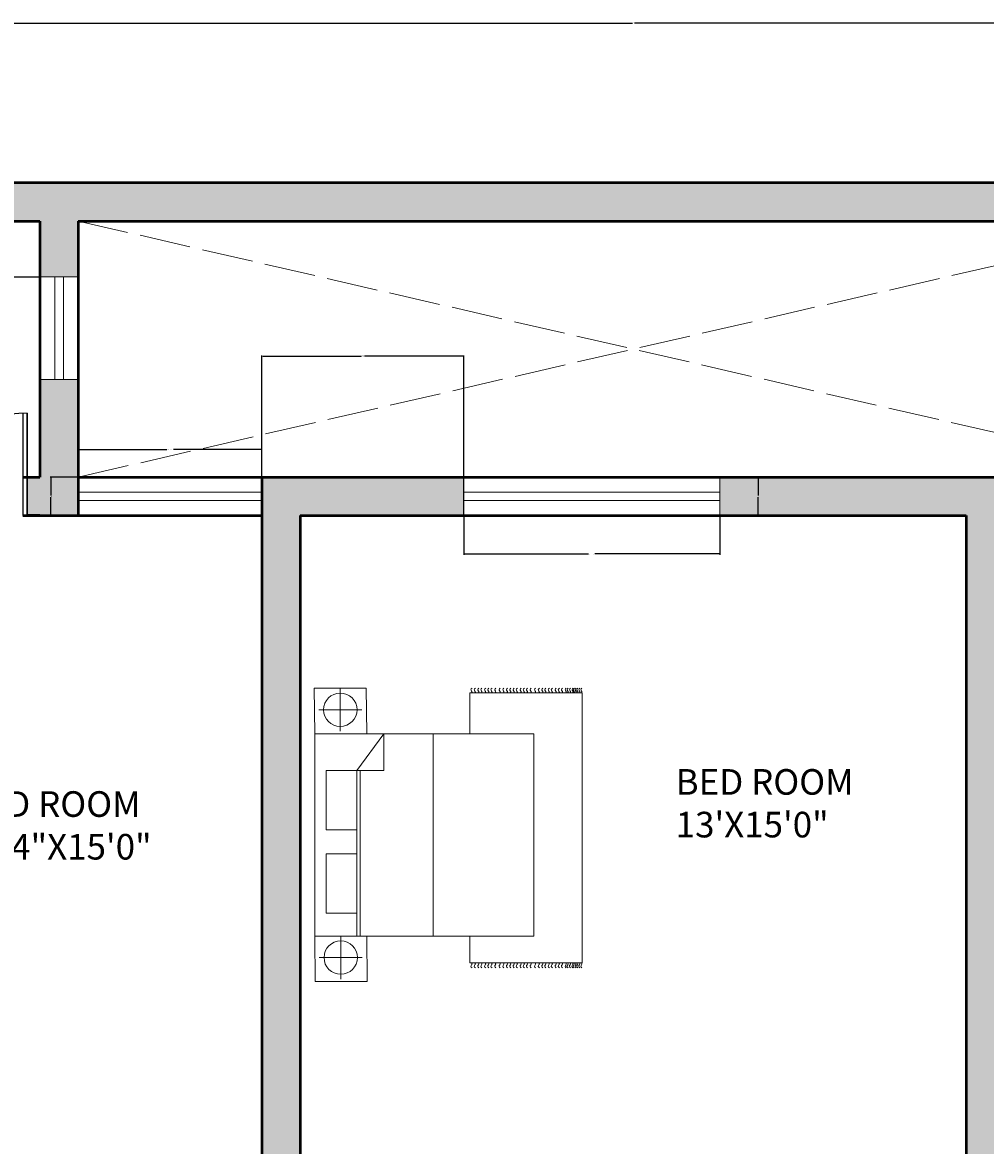
# Model space of a CAD drawing. Units: inches. Extents: x 383 to 970, y 275 to 1088.
# Tile 8 of 11: x 533 to 759, y 825 to 1088. Entities that reach past the tile are written whole.
import ezdxf

# ---------------------------------------------------------------- set-up
doc = ezdxf.new("R2010")
doc.units = ezdxf.units.IN
doc.header["$MEASUREMENT"] = 0
doc.linetypes.add('ACAD_ISO02W100', pattern=[15, 12, -3])
for name, color, linetype, lineweight in [('A-ANNO-DIMS', 2, 'Continuous', 18), ('A-AREA-IDEN', 7, 'Continuous', 18), ('A-DOOR', 3, 'Continuous', 25), ('A-FLOR-OPEN', 8, 'ACAD_ISO02W100', 13), ('A-FURN', 8, 'Continuous', 18), ('A-GLAZ', 4, 'Continuous', 18), ('A-WALL', 7, 'Continuous', 50)]:
    doc.layers.add(name, color=color, linetype=linetype, lineweight=lineweight)
doc.layers.add('A-WALL-PATT', color=251, linetype='Continuous', lineweight=13, true_color=0x636466)
doc.styles.get("Standard").update_dxf_attribs({"font": 'arial.ttf'})
doc.dimstyles.get("Standard").update_dxf_attribs({"dimtxt": 0.18, "dimasz": 0.18, "dimexe": 0.18, "dimexo": 0.0625, "dimgap": 0.09, "dimtad": 0, "dimtih": 1, "dimtoh": 1, "dimdec": 4, "dimzin": 0, "dimdsep": 46, "dimtxsty": 'Standard', "dimcen": 0.09, "dimadec": 0, "dimazin": 0, "dimtfac": 1, "dimtdec": 4, "dimtofl": 0, "dimtmove": 0, "dimatfit": 3, "dimfxl": 1, "dimtolj": 1, "dimtzin": 0, "dimarcsym": 0})

# ---------------------------------------------------------------- blocks, each defined once
blk = doc.blocks.new('BED-DOUBLE-WITH-NIGHTSTANDS')
for p, q in [((6.09, 68.68), (6.09, 58.62)), ((36.42, 67.59), (62.78, 67.59)), ((36.42, 58.05), (36.42, 67.59)), ((62.78, 67.59), (62.78, 4.35)), ((1.07, 63.65), (11.12, 63.65)), ((9.97, 49.39), (16.32, 58)), ((16.32, 49.44), (16.32, 58)), ((27.82, 58.05), (27.82, 10.63)), ((9.97, 49.44), (16.32, 49.44)), ((9.97, 49.39), (9.97, 10.63)), ((10.78, 49.44), (10.78, 10.63)), ((6.2, 10.63), (6.2, 0.57)), ((36.42, 4.35), (36.42, 10.65)), ((1.17, 5.6), (11.22, 5.6)), ((62.78, 4.35), (36.42, 4.35))]:
    blk.add_line(p, q)
for points in [[(12.29, 58.05), (12.19, 68.68), (0, 68.68), (0.1, 58.05)], [(0.1, 58.05), (51.42, 58.05), (51.42, 10.63), (0.1, 10.63)], [(2.8, 49.44), (9.97, 49.44), (9.97, 35.55), (2.8, 35.55)], [(2.8, 29.88), (9.97, 29.88), (9.97, 15.98), (2.8, 15.98)], [(12.39, 0), (12.29, 10.63), (0.1, 10.63), (0.21, 0)]]:
    blk.add_lwpolyline(points, close=True)
for centre in [(6.09, 63.65), (6.2, 5.6)]:
    blk.add_circle(centre, 3.92)
for points, knots in [([(36.95, 68.71), (36.83, 68.61), (36.59, 68.42), (36.83, 68.08), (37, 67.8), (36.89, 67.65), (36.85, 67.58)], [0, 0, 0, 0, 0.400747, 0.791423, 1.067667, 1.29709, 1.29709, 1.29709, 1.29709]), ([(37.73, 68.71), (37.61, 68.61), (37.37, 68.42), (37.61, 68.08), (37.78, 67.8), (37.67, 67.65), (37.62, 67.58)], [0, 0, 0, 0, 0.400747, 0.791423, 1.067667, 1.29709, 1.29709, 1.29709, 1.29709]), ([(38.54, 68.71), (38.42, 68.61), (38.18, 68.42), (38.42, 68.08), (38.59, 67.8), (38.49, 67.65), (38.44, 67.58)], [0, 0, 0, 0, 0.400747, 0.791423, 1.067667, 1.29709, 1.29709, 1.29709, 1.29709]), ([(39.27, 68.71), (39.15, 68.61), (38.91, 68.42), (39.15, 68.08), (39.32, 67.8), (39.22, 67.65), (39.17, 67.58)], [0, 0, 0, 0, 0.400747, 0.791423, 1.067667, 1.29709, 1.29709, 1.29709, 1.29709]), ([(40.15, 68.71), (40.03, 68.61), (39.79, 68.42), (40.03, 68.08), (40.21, 67.8), (40.1, 67.65), (40.05, 67.58)], [0, 0, 0, 0, 0.400747, 0.791423, 1.067667, 1.29709, 1.29709, 1.29709, 1.29709]), ([(40.91, 68.71), (40.78, 68.61), (40.54, 68.42), (40.78, 68.08), (40.96, 67.8), (40.85, 67.65), (40.8, 67.58)], [0, 0, 0, 0, 0.400747, 0.791423, 1.067667, 1.29709, 1.29709, 1.29709, 1.29709]), ([(41.63, 68.71), (41.51, 68.61), (41.27, 68.42), (41.51, 68.08), (41.69, 67.8), (41.58, 67.65), (41.53, 67.58)], [0, 0, 0, 0, 0.400747, 0.791423, 1.067667, 1.29709, 1.29709, 1.29709, 1.29709]), ([(42.52, 68.71), (42.39, 68.61), (42.16, 68.42), (42.39, 68.08), (42.57, 67.8), (42.46, 67.65), (42.41, 67.58)], [0, 0, 0, 0, 0.400747, 0.791423, 1.067667, 1.29709, 1.29709, 1.29709, 1.29709]), ([(43.55, 68.71), (43.43, 68.61), (43.19, 68.42), (43.43, 68.08), (43.6, 67.8), (43.5, 67.65), (43.45, 67.58)], [0, 0, 0, 0, 0.400747, 0.791423, 1.067667, 1.29709, 1.29709, 1.29709, 1.29709]), ([(44.43, 68.71), (44.31, 68.61), (44.07, 68.42), (44.31, 68.08), (44.49, 67.8), (44.38, 67.65), (44.33, 67.58)], [0, 0, 0, 0, 0.400747, 0.791423, 1.067667, 1.29709, 1.29709, 1.29709, 1.29709]), ([(45.25, 68.71), (45.13, 68.61), (44.89, 68.42), (45.13, 68.08), (45.3, 67.8), (45.2, 67.65), (45.15, 67.58)], [0, 0, 0, 0, 0.400747, 0.791423, 1.067667, 1.29709, 1.29709, 1.29709, 1.29709]), ([(46.03, 68.71), (45.91, 68.61), (45.67, 68.42), (45.91, 68.08), (46.08, 67.8), (45.97, 67.65), (45.92, 67.58)], [0, 0, 0, 0, 0.400747, 0.791423, 1.067667, 1.29709, 1.29709, 1.29709, 1.29709]), ([(46.84, 68.71), (46.72, 68.61), (46.48, 68.42), (46.72, 68.08), (46.9, 67.8), (46.79, 67.65), (46.74, 67.58)], [0, 0, 0, 0, 0.400747, 0.791423, 1.067667, 1.29709, 1.29709, 1.29709, 1.29709]), ([(47.57, 68.71), (47.45, 68.61), (47.21, 68.42), (47.45, 68.08), (47.62, 67.8), (47.52, 67.65), (47.47, 67.58)], [0, 0, 0, 0, 0.400747, 0.791423, 1.067667, 1.29709, 1.29709, 1.29709, 1.29709]), ([(48.45, 68.71), (48.33, 68.61), (48.09, 68.42), (48.33, 68.08), (48.51, 67.8), (48.4, 67.65), (48.35, 67.58)], [0, 0, 0, 0, 0.400747, 0.791423, 1.067667, 1.29709, 1.29709, 1.29709, 1.29709]), ([(49.21, 68.71), (49.08, 68.61), (48.85, 68.42), (49.08, 68.08), (49.26, 67.8), (49.15, 67.65), (49.1, 67.58)], [0, 0, 0, 0, 0.400747, 0.791423, 1.067667, 1.29709, 1.29709, 1.29709, 1.29709]), ([(49.93, 68.71), (49.81, 68.61), (49.57, 68.42), (49.81, 68.08), (49.99, 67.8), (49.88, 67.65), (49.83, 67.58)], [0, 0, 0, 0, 0.400747, 0.791423, 1.067667, 1.29709, 1.29709, 1.29709, 1.29709]), ([(50.82, 68.71), (50.69, 68.61), (50.46, 68.42), (50.69, 68.08), (50.87, 67.8), (50.76, 67.65), (50.71, 67.58)], [0, 0, 0, 0, 0.400747, 0.791423, 1.067667, 1.29709, 1.29709, 1.29709, 1.29709]), ([(51.85, 68.71), (51.73, 68.61), (51.49, 68.42), (51.73, 68.08), (51.9, 67.8), (51.8, 67.65), (51.75, 67.58)], [0, 0, 0, 0, 0.400747, 0.791423, 1.067667, 1.29709, 1.29709, 1.29709, 1.29709]), ([(52.74, 68.71), (52.61, 68.61), (52.37, 68.42), (52.61, 68.08), (52.79, 67.8), (52.68, 67.65), (52.63, 67.58)], [0, 0, 0, 0, 0.400747, 0.791423, 1.067667, 1.29709, 1.29709, 1.29709, 1.29709]), ([(53.55, 68.71), (53.43, 68.61), (53.19, 68.42), (53.43, 68.08), (53.6, 67.8), (53.5, 67.65), (53.45, 67.58)], [0, 0, 0, 0, 0.400747, 0.791423, 1.067667, 1.29709, 1.29709, 1.29709, 1.29709]), ([(54.24, 68.71), (54.12, 68.61), (53.88, 68.42), (54.12, 68.08), (54.29, 67.8), (54.19, 67.65), (54.14, 67.58)], [0, 0, 0, 0, 0.400747, 0.791423, 1.067667, 1.29709, 1.29709, 1.29709, 1.29709]), ([(55.06, 68.71), (54.94, 68.61), (54.7, 68.42), (54.94, 68.08), (55.11, 67.8), (55, 67.65), (54.95, 67.58)], [0, 0, 0, 0, 0.400747, 0.791423, 1.067667, 1.29709, 1.29709, 1.29709, 1.29709]), ([(55.78, 68.71), (55.66, 68.61), (55.42, 68.42), (55.66, 68.08), (55.84, 67.8), (55.73, 67.65), (55.68, 67.58)], [0, 0, 0, 0, 0.400747, 0.791423, 1.067667, 1.29709, 1.29709, 1.29709, 1.29709]), ([(56.67, 68.71), (56.55, 68.61), (56.31, 68.42), (56.55, 68.08), (56.72, 67.8), (56.61, 67.65), (56.56, 67.58)], [0, 0, 0, 0, 0.400747, 0.791423, 1.067667, 1.29709, 1.29709, 1.29709, 1.29709]), ([(57.42, 68.71), (57.3, 68.61), (57.06, 68.42), (57.3, 68.08), (57.47, 67.8), (57.36, 67.65), (57.32, 67.58)], [0, 0, 0, 0, 0.400747, 0.791423, 1.067667, 1.29709, 1.29709, 1.29709, 1.29709]), ([(58.15, 68.71), (58.03, 68.61), (57.79, 68.42), (58.03, 68.08), (58.2, 67.8), (58.1, 67.66), (58.05, 67.59)], [0, 0, 0, 0, 0.400747, 0.791423, 1.067667, 1.283686, 1.283686, 1.283686, 1.283686]), ([(59.03, 68.71), (58.91, 68.61), (58.67, 68.42), (58.91, 68.08), (59.08, 67.8), (58.98, 67.66), (58.93, 67.59)], [0, 0, 0, 0, 0.400747, 0.791423, 1.067667, 1.283686, 1.283686, 1.283686, 1.283686]), ([(59.46, 68.71), (59.34, 68.61), (59.09, 68.42), (59.34, 68.08), (59.51, 67.8), (59.41, 67.66), (59.36, 67.59)], [0, 0, 0, 0, 0.402903, 0.794912, 1.071156, 1.287177, 1.287177, 1.287177, 1.287177]), ([(60.05, 68.71), (59.93, 68.61), (59.69, 68.42), (59.93, 68.08), (60.1, 67.8), (60, 67.66), (59.96, 67.59)], [0, 0, 0, 0, 0.400747, 0.791423, 1.067667, 1.283686, 1.283686, 1.283686, 1.283686]), ([(60.63, 68.71), (60.51, 68.61), (60.27, 68.42), (60.51, 68.08), (60.68, 67.8), (60.58, 67.66), (60.53, 67.59)], [0, 0, 0, 0, 0.400747, 0.791423, 1.067667, 1.283686, 1.283686, 1.283686, 1.283686]), ([(60.94, 68.71), (60.82, 68.61), (60.58, 68.42), (60.81, 68.08), (60.99, 67.8), (60.89, 67.66), (60.84, 67.59)], [0, 0, 0, 0, 0.400747, 0.791423, 1.067667, 1.283686, 1.283686, 1.283686, 1.283686]), ([(61.36, 68.71), (61.23, 68.61), (60.99, 68.42), (61.23, 68.08), (61.41, 67.8), (61.3, 67.65), (61.25, 67.58)], [0, 0, 0, 0, 0.400747, 0.791423, 1.067667, 1.29709, 1.29709, 1.29709, 1.29709]), ([(61.75, 68.71), (61.63, 68.61), (61.39, 68.42), (61.63, 68.08), (61.8, 67.8), (61.7, 67.65), (61.65, 67.58)], [0, 0, 0, 0, 0.400747, 0.791423, 1.067667, 1.29709, 1.29709, 1.29709, 1.29709]), ([(62.24, 68.71), (62.12, 68.61), (61.88, 68.42), (62.12, 68.08), (62.29, 67.8), (62.18, 67.65), (62.13, 67.58)], [0, 0, 0, 0, 0.400747, 0.791423, 1.067667, 1.29709, 1.29709, 1.29709, 1.29709]), ([(62.71, 68.71), (62.59, 68.61), (62.35, 68.42), (62.59, 68.08), (62.76, 67.8), (62.66, 67.65), (62.61, 67.58)], [0, 0, 0, 0, 0.400747, 0.791423, 1.067667, 1.29709, 1.29709, 1.29709, 1.29709]), ([(36.95, 3.23), (36.83, 3.32), (36.59, 3.52), (36.83, 3.86), (37, 4.14), (36.89, 4.29), (36.85, 4.35)], [0, 0, 0, 0, 0.400747, 0.791423, 1.067667, 1.29709, 1.29709, 1.29709, 1.29709]), ([(37.73, 3.23), (37.61, 3.32), (37.37, 3.52), (37.61, 3.86), (37.78, 4.14), (37.67, 4.29), (37.62, 4.35)], [0, 0, 0, 0, 0.400747, 0.791423, 1.067667, 1.29709, 1.29709, 1.29709, 1.29709]), ([(38.54, 3.23), (38.42, 3.32), (38.18, 3.52), (38.42, 3.86), (38.59, 4.14), (38.49, 4.29), (38.44, 4.35)], [0, 0, 0, 0, 0.400747, 0.791423, 1.067667, 1.29709, 1.29709, 1.29709, 1.29709]), ([(39.27, 3.23), (39.15, 3.32), (38.91, 3.52), (39.15, 3.86), (39.32, 4.14), (39.22, 4.29), (39.17, 4.35)], [0, 0, 0, 0, 0.400747, 0.791423, 1.067667, 1.29709, 1.29709, 1.29709, 1.29709]), ([(40.15, 3.23), (40.03, 3.32), (39.79, 3.52), (40.03, 3.86), (40.21, 4.14), (40.1, 4.29), (40.05, 4.35)], [0, 0, 0, 0, 0.400747, 0.791423, 1.067667, 1.29709, 1.29709, 1.29709, 1.29709]), ([(40.91, 3.23), (40.78, 3.32), (40.54, 3.52), (40.78, 3.86), (40.96, 4.14), (40.85, 4.29), (40.8, 4.35)], [0, 0, 0, 0, 0.400747, 0.791423, 1.067667, 1.29709, 1.29709, 1.29709, 1.29709]), ([(41.63, 3.23), (41.51, 3.32), (41.27, 3.52), (41.51, 3.86), (41.69, 4.14), (41.58, 4.29), (41.53, 4.35)], [0, 0, 0, 0, 0.400747, 0.791423, 1.067667, 1.29709, 1.29709, 1.29709, 1.29709]), ([(42.52, 3.23), (42.39, 3.32), (42.16, 3.52), (42.39, 3.86), (42.57, 4.14), (42.46, 4.29), (42.41, 4.35)], [0, 0, 0, 0, 0.400747, 0.791423, 1.067667, 1.29709, 1.29709, 1.29709, 1.29709]), ([(43.55, 3.23), (43.43, 3.32), (43.19, 3.52), (43.43, 3.86), (43.6, 4.14), (43.5, 4.29), (43.45, 4.35)], [0, 0, 0, 0, 0.400747, 0.791423, 1.067667, 1.29709, 1.29709, 1.29709, 1.29709]), ([(44.43, 3.23), (44.31, 3.32), (44.07, 3.52), (44.31, 3.86), (44.49, 4.14), (44.38, 4.29), (44.33, 4.35)], [0, 0, 0, 0, 0.400747, 0.791423, 1.067667, 1.29709, 1.29709, 1.29709, 1.29709]), ([(45.25, 3.23), (45.13, 3.32), (44.89, 3.52), (45.13, 3.86), (45.3, 4.14), (45.2, 4.29), (45.15, 4.35)], [0, 0, 0, 0, 0.400747, 0.791423, 1.067667, 1.29709, 1.29709, 1.29709, 1.29709]), ([(46.03, 3.23), (45.91, 3.32), (45.67, 3.52), (45.91, 3.86), (46.08, 4.14), (45.97, 4.29), (45.92, 4.35)], [0, 0, 0, 0, 0.400747, 0.791423, 1.067667, 1.29709, 1.29709, 1.29709, 1.29709]), ([(46.84, 3.23), (46.72, 3.32), (46.48, 3.52), (46.72, 3.86), (46.9, 4.14), (46.79, 4.29), (46.74, 4.35)], [0, 0, 0, 0, 0.400747, 0.791423, 1.067667, 1.29709, 1.29709, 1.29709, 1.29709]), ([(47.57, 3.23), (47.45, 3.32), (47.21, 3.52), (47.45, 3.86), (47.62, 4.14), (47.52, 4.29), (47.47, 4.35)], [0, 0, 0, 0, 0.400747, 0.791423, 1.067667, 1.29709, 1.29709, 1.29709, 1.29709]), ([(48.45, 3.23), (48.33, 3.32), (48.09, 3.52), (48.33, 3.86), (48.51, 4.14), (48.4, 4.29), (48.35, 4.35)], [0, 0, 0, 0, 0.400747, 0.791423, 1.067667, 1.29709, 1.29709, 1.29709, 1.29709]), ([(49.21, 3.23), (49.08, 3.32), (48.85, 3.52), (49.08, 3.86), (49.26, 4.14), (49.15, 4.29), (49.1, 4.35)], [0, 0, 0, 0, 0.400747, 0.791423, 1.067667, 1.29709, 1.29709, 1.29709, 1.29709]), ([(49.93, 3.23), (49.81, 3.32), (49.57, 3.52), (49.81, 3.86), (49.99, 4.14), (49.88, 4.29), (49.83, 4.35)], [0, 0, 0, 0, 0.400747, 0.791423, 1.067667, 1.29709, 1.29709, 1.29709, 1.29709]), ([(50.82, 3.23), (50.69, 3.32), (50.46, 3.52), (50.69, 3.86), (50.87, 4.14), (50.76, 4.29), (50.71, 4.35)], [0, 0, 0, 0, 0.400747, 0.791423, 1.067667, 1.29709, 1.29709, 1.29709, 1.29709]), ([(51.85, 3.23), (51.73, 3.32), (51.49, 3.52), (51.73, 3.86), (51.9, 4.14), (51.8, 4.29), (51.75, 4.35)], [0, 0, 0, 0, 0.400747, 0.791423, 1.067667, 1.29709, 1.29709, 1.29709, 1.29709]), ([(52.74, 3.23), (52.61, 3.32), (52.37, 3.52), (52.61, 3.86), (52.79, 4.14), (52.68, 4.29), (52.63, 4.35)], [0, 0, 0, 0, 0.400747, 0.791423, 1.067667, 1.29709, 1.29709, 1.29709, 1.29709]), ([(53.55, 3.23), (53.43, 3.32), (53.19, 3.52), (53.43, 3.86), (53.6, 4.14), (53.5, 4.29), (53.45, 4.35)], [0, 0, 0, 0, 0.400747, 0.791423, 1.067667, 1.29709, 1.29709, 1.29709, 1.29709]), ([(54.24, 3.23), (54.12, 3.32), (53.88, 3.52), (54.12, 3.86), (54.29, 4.14), (54.19, 4.29), (54.14, 4.35)], [0, 0, 0, 0, 0.400747, 0.791423, 1.067667, 1.29709, 1.29709, 1.29709, 1.29709]), ([(55.06, 3.23), (54.94, 3.32), (54.7, 3.52), (54.94, 3.86), (55.11, 4.14), (55, 4.29), (54.95, 4.35)], [0, 0, 0, 0, 0.400747, 0.791423, 1.067667, 1.29709, 1.29709, 1.29709, 1.29709]), ([(55.78, 3.23), (55.66, 3.32), (55.42, 3.52), (55.66, 3.86), (55.84, 4.14), (55.73, 4.29), (55.68, 4.35)], [0, 0, 0, 0, 0.400747, 0.791423, 1.067667, 1.29709, 1.29709, 1.29709, 1.29709]), ([(56.67, 3.23), (56.55, 3.32), (56.31, 3.52), (56.55, 3.86), (56.72, 4.14), (56.61, 4.29), (56.56, 4.35)], [0, 0, 0, 0, 0.400747, 0.791423, 1.067667, 1.29709, 1.29709, 1.29709, 1.29709]), ([(57.42, 3.23), (57.3, 3.32), (57.06, 3.52), (57.3, 3.86), (57.47, 4.14), (57.36, 4.29), (57.32, 4.35)], [0, 0, 0, 0, 0.400747, 0.791423, 1.067667, 1.29709, 1.29709, 1.29709, 1.29709]), ([(58.15, 3.23), (58.03, 3.32), (57.79, 3.52), (58.03, 3.86), (58.2, 4.14), (58.09, 4.29), (58.04, 4.35)], [0, 0, 0, 0, 0.400747, 0.791423, 1.067667, 1.29709, 1.29709, 1.29709, 1.29709]), ([(59.03, 3.23), (58.91, 3.32), (58.67, 3.52), (58.91, 3.86), (59.08, 4.14), (58.98, 4.29), (58.93, 4.35)], [0, 0, 0, 0, 0.400747, 0.791423, 1.067667, 1.29709, 1.29709, 1.29709, 1.29709]), ([(59.46, 3.23), (59.33, 3.32), (59.08, 3.52), (59.34, 3.86), (59.51, 4.14), (59.4, 4.29), (59.36, 4.35)], [0, 0, 0, 0, 0.407265, 0.802015, 1.07826, 1.307683, 1.307683, 1.307683, 1.307683]), ([(60.03, 3.23), (59.9, 3.32), (59.67, 3.52), (59.9, 3.86), (60.08, 4.14), (59.97, 4.29), (59.92, 4.35)], [0, 0, 0, 0, 0.400747, 0.791423, 1.067667, 1.29709, 1.29709, 1.29709, 1.29709]), ([(60.6, 3.23), (60.48, 3.32), (60.24, 3.52), (60.48, 3.86), (60.65, 4.14), (60.54, 4.29), (60.5, 4.35)], [0, 0, 0, 0, 0.400747, 0.791423, 1.067667, 1.29709, 1.29709, 1.29709, 1.29709]), ([(60.91, 3.23), (60.79, 3.32), (60.55, 3.52), (60.79, 3.86), (60.96, 4.14), (60.85, 4.29), (60.81, 4.35)], [0, 0, 0, 0, 0.400747, 0.791423, 1.067667, 1.29709, 1.29709, 1.29709, 1.29709]), ([(61.33, 3.23), (61.21, 3.32), (60.97, 3.52), (61.21, 3.86), (61.38, 4.14), (61.27, 4.29), (61.22, 4.35)], [0, 0, 0, 0, 0.400747, 0.791423, 1.067667, 1.29709, 1.29709, 1.29709, 1.29709]), ([(61.72, 3.23), (61.6, 3.32), (61.36, 3.52), (61.6, 3.86), (61.78, 4.14), (61.67, 4.29), (61.62, 4.35)], [0, 0, 0, 0, 0.400747, 0.791423, 1.067667, 1.29709, 1.29709, 1.29709, 1.29709]), ([(62.21, 3.23), (62.09, 3.32), (61.85, 3.52), (62.09, 3.86), (62.26, 4.14), (62.16, 4.29), (62.11, 4.35)], [0, 0, 0, 0, 0.400747, 0.791423, 1.067667, 1.29709, 1.29709, 1.29709, 1.29709]), ([(62.71, 3.23), (62.59, 3.32), (62.35, 3.52), (62.59, 3.86), (62.76, 4.14), (62.66, 4.29), (62.61, 4.35)], [0, 0, 0, 0, 0.400747, 0.791423, 1.067667, 1.29709, 1.29709, 1.29709, 1.29709])]:
    blk.add_open_spline(points, degree=3, knots=knots)
blk = doc.blocks.new('DOOR-LEAF-24IN')
for p, q in [((23, 24), (23, 0)), ((24, 0), (24, 24)), ((24, 0), (23, 0))]:
    blk.add_line(p, q)
blk.add_arc((24, -2.7), 26.7, 90, 154.0108)
blk = doc.blocks.new('WIN-VENT-24IN')
for p, q in [((0, 0), (0, 24)), ((3.5, 0), (3.5, 24)), ((5.5, 24), (5.5, 0)), ((9, 24), (9, 0))]:
    blk.add_line(p, q)
blk = doc.blocks.new('WIN-60IN')
for p, q in [((60, 9), (0, 9)), ((60, 5.5), (0, 5.5)), ((0, 3.5), (60, 3.5)), ((0, 0), (60, 0))]:
    blk.add_line(p, q)
blk = doc.blocks.new('WIN-43IN')
for p, q in [((43, 9), (0, 9)), ((43, 5.5), (0, 5.5)), ((0, 3.5), (43, 3.5)), ((0, 0), (43, 0))]:
    blk.add_line(p, q)
blk = doc.blocks.new('*D21')
at = {"layer": 'A-ANNO-DIMS', "color": 0, "lineweight": -2, "transparency": 16777216}
for p, q in [((636.51, 972.07), (636.51, 962.96)), ((696.51, 972.07), (696.51, 962.96)), ((636.69, 963.14), (665.75, 963.14)), ((696.33, 963.14), (667.26, 963.14))]:
    blk.add_line(p, q, dxfattribs=at)
at = {"layer": 'A-ANNO-DIMS', "color": 0, "transparency": 16777216}
for points in [[(636.69, 963.17), (636.69, 963.11), (636.51, 963.14)], [(696.33, 963.17), (696.33, 963.11), (696.51, 963.14)]]:
    blk.add_solid(points, dxfattribs=at)
at = {"layer": 'Defpoints', "color": 0, "transparency": 16777216}
for p in [(636.51, 972.14), (696.51, 972.14), (696.51, 963.14)]:
    blk.add_point(p, dxfattribs=at)
at = {"layer": 'A-ANNO-DIMS', "color": 0, "transparency": 16777216, "insert": (666.51, 963.14), "char_height": 0.18, "attachment_point": 5}
blk.add_mtext('\\A1;W1 60 TYP.', dxfattribs=at)
blk = doc.blocks.new('*D22')
at = {"layer": 'A-ANNO-DIMS', "color": 0, "lineweight": -2, "transparency": 16777216}
for p, q in [((696.57, 981.14), (705.69, 981.14)), ((705.51, 980.96), (705.51, 976.82)), ((705.51, 972.32), (705.51, 976.45)), ((696.57, 972.14), (705.69, 972.14))]:
    blk.add_line(p, q, dxfattribs=at)
at = {"layer": 'A-ANNO-DIMS', "color": 0, "transparency": 16777216}
for points in [[(705.48, 980.96), (705.54, 980.96), (705.51, 981.14)], [(705.48, 972.32), (705.54, 972.32), (705.51, 972.14)]]:
    blk.add_solid(points, dxfattribs=at)
at = {"layer": 'Defpoints', "color": 0, "transparency": 16777216}
for p in [(696.51, 981.14), (705.51, 981.14), (696.51, 972.14)]:
    blk.add_point(p, dxfattribs=at)
at = {"layer": 'A-ANNO-DIMS', "color": 0, "transparency": 16777216, "insert": (705.51, 976.64), "char_height": 0.18, "attachment_point": 5}
blk.add_mtext('\\A1;9 TYP.', dxfattribs=at)
blk = doc.blocks.new('*D23')
at = {"layer": 'A-ANNO-DIMS', "color": 0, "lineweight": -2, "transparency": 16777216}
for p, q in [((546.24, 981.2), (546.24, 987.77)), ((546.42, 987.59), (566.98, 987.59)), ((589.06, 987.59), (568.5, 987.59)), ((589.24, 981.2), (589.24, 987.77))]:
    blk.add_line(p, q, dxfattribs=at)
at = {"layer": 'A-ANNO-DIMS', "color": 0, "transparency": 16777216}
for points in [[(546.42, 987.62), (546.42, 987.56), (546.24, 987.59)], [(589.06, 987.62), (589.06, 987.56), (589.24, 987.59)]]:
    blk.add_solid(points, dxfattribs=at)
at = {"layer": 'Defpoints', "color": 0, "transparency": 16777216}
for p in [(589.24, 987.59), (546.24, 981.14), (589.24, 981.14)]:
    blk.add_point(p, dxfattribs=at)
at = {"layer": 'A-ANNO-DIMS', "color": 0, "transparency": 16777216, "insert": (567.74, 987.59), "char_height": 0.18, "attachment_point": 5}
blk.add_mtext('\\A1;W2 43 TYP.', dxfattribs=at)
blk = doc.blocks.new('*D24')
at = {"layer": 'A-ANNO-DIMS', "color": 0, "lineweight": -2, "transparency": 16777216}
for p, q in [((546.18, 981.14), (539.61, 981.14)), ((539.79, 980.96), (539.79, 976.82)), ((539.79, 972.32), (539.79, 976.45)), ((546.18, 972.14), (539.61, 972.14))]:
    blk.add_line(p, q, dxfattribs=at)
at = {"layer": 'A-ANNO-DIMS', "color": 0, "transparency": 16777216}
for points in [[(539.76, 980.96), (539.82, 980.96), (539.79, 981.14)], [(539.76, 972.32), (539.82, 972.32), (539.79, 972.14)]]:
    blk.add_solid(points, dxfattribs=at)
at = {"layer": 'Defpoints', "color": 0, "transparency": 16777216}
for p in [(539.79, 981.14), (546.24, 981.14), (546.24, 972.14)]:
    blk.add_point(p, dxfattribs=at)
at = {"layer": 'A-ANNO-DIMS', "color": 0, "transparency": 16777216, "insert": (539.79, 976.64), "char_height": 0.18, "attachment_point": 5}
blk.add_mtext('\\A1;9 TYP.', dxfattribs=at)
blk = doc.blocks.new('*D37')
at = {"layer": 'A-ANNO-DIMS', "color": 0, "lineweight": -2, "transparency": 16777216}
for p, q in [((420.24, 1050.2), (420.24, 1087.67)), ((420.42, 1087.49), (675.95, 1087.49)), ((932.06, 1087.49), (676.53, 1087.49)), ((932.24, 1050.2), (932.24, 1087.67))]:
    blk.add_line(p, q, dxfattribs=at)
at = {"layer": 'A-ANNO-DIMS', "color": 0, "transparency": 16777216}
for points in [[(420.42, 1087.52), (420.42, 1087.46), (420.24, 1087.49)], [(932.06, 1087.52), (932.06, 1087.46), (932.24, 1087.49)]]:
    blk.add_solid(points, dxfattribs=at)
at = {"layer": 'Defpoints', "color": 0, "transparency": 16777216}
for p in [(932.24, 1087.49), (420.24, 1050.14), (932.24, 1050.14)]:
    blk.add_point(p, dxfattribs=at)
at = {"layer": 'A-ANNO-DIMS', "color": 0, "transparency": 16777216, "insert": (676.24, 1087.49), "char_height": 0.18, "attachment_point": 5}
blk.add_mtext('\\A1;512', dxfattribs=at)
blk = doc.blocks.new('*D52')
at = {"layer": 'A-ANNO-DIMS', "color": 0, "lineweight": -2, "transparency": 16777216}
for p, q in [((589.24, 972.2), (589.24, 1009.67)), ((589.42, 1009.49), (612.48, 1009.49)), ((636.33, 1009.49), (613.27, 1009.49)), ((636.51, 972.2), (636.51, 1009.67))]:
    blk.add_line(p, q, dxfattribs=at)
at = {"layer": 'A-ANNO-DIMS', "color": 0, "transparency": 16777216}
for points in [[(589.42, 1009.52), (589.42, 1009.46), (589.24, 1009.49)], [(636.33, 1009.52), (636.33, 1009.46), (636.51, 1009.49)]]:
    blk.add_solid(points, dxfattribs=at)
at = {"layer": 'Defpoints', "color": 0, "transparency": 16777216}
for p in [(636.51, 1009.49), (589.24, 972.14), (636.51, 972.14)]:
    blk.add_point(p, dxfattribs=at)
at = {"layer": 'A-ANNO-DIMS', "color": 0, "transparency": 16777216, "insert": (612.87, 1009.49), "char_height": 0.18, "attachment_point": 5}
blk.add_mtext('\\A1;47.27', dxfattribs=at)
blk = doc.blocks.new('*D62')
at = {"layer": 'A-ANNO-DIMS', "color": 0, "lineweight": -2, "transparency": 16777216}
for p, q in [((537.18, 1041.14), (499.71, 1041.14)), ((499.89, 1040.96), (499.89, 1034.77)), ((499.89, 1028.21), (499.89, 1034.4)), ((537.18, 1028.03), (499.71, 1028.03))]:
    blk.add_line(p, q, dxfattribs=at)
at = {"layer": 'A-ANNO-DIMS', "color": 0, "transparency": 16777216}
for points in [[(499.86, 1040.96), (499.92, 1040.96), (499.89, 1041.14)], [(499.86, 1028.21), (499.92, 1028.21), (499.89, 1028.03)]]:
    blk.add_solid(points, dxfattribs=at)
at = {"layer": 'Defpoints', "color": 0, "transparency": 16777216}
for p in [(499.89, 1041.14), (537.24, 1041.14), (537.24, 1028.03)]:
    blk.add_point(p, dxfattribs=at)
at = {"layer": 'A-ANNO-DIMS', "color": 0, "transparency": 16777216, "insert": (499.89, 1034.59), "char_height": 0.18, "attachment_point": 5}
blk.add_mtext('\\A1;13.103', dxfattribs=at)

msp = doc.modelspace()

# ---------------------------------------------------------------- hatches: boundary and pattern name
at = {"layer": 'A-WALL-PATT'}
h = msp.add_hatch(color=256, dxfattribs=at)
h.dxf.hatch_style = 1
h.paths.add_polyline_path([(651.24, 321.1365), (651.24, 417.1365), (735.24, 417.1365), (735.24, 491.9233), (726.24, 491.9233), (726.24, 426.1365), (582.24, 426.1365), (582.24, 606.1365), (687.24, 606.1365), (687.24, 615.1365), (573.24, 615.1365), (573.24, 546.1365), (570.24, 546.1365), (570.24, 537.1365), (573.24, 537.1365), (573.24, 414.1365), (582.24, 414.1365), (582.24, 417.1365), (642.24, 417.1365), (642.24, 321.1365), (621.6203, 321.1365), (621.6203, 312.1365), (651.24, 312.1365)], flags=17)
h.paths.add_polyline_path([(597.6203, 321.1365), (582.24, 321.1365), (582.24, 390.1365), (573.24, 390.1365), (573.24, 321.1365), (570.24, 321.1365), (570.24, 312.1365), (573.24, 312.1365), (597.6203, 312.1365)], flags=16)
h.paths.add_polyline_path([(534.24, 321.1365), (500.8868, 321.1365), (500.8868, 312.1365), (534.24, 312.1365)], flags=17)
h.paths.add_polyline_path([(735.24, 606.1365), (738.24, 606.1365), (738.24, 615.1365), (723.24, 615.1365), (723.24, 606.1365), (726.24, 606.1365), (726.24, 551.9233), (735.24, 551.9233)], flags=17)
h.paths.add_polyline_path([(848.0899, 615.1365), (814.24, 615.1365), (814.24, 689.38), (805.24, 689.38), (805.24, 615.1365), (802.24, 615.1365), (802.24, 606.1365), (848.0899, 606.1365)], flags=17)
h.paths.add_polyline_path([(530.24, 615.1365), (498.24, 615.1365), (498.24, 646.5351), (489.24, 646.5351), (489.24, 615.1365), (466.771, 615.1365), (466.771, 606.1365), (521.24, 606.1365), (521.24, 603.1365), (530.24, 603.1365), (530.24, 606.1365)], flags=17)
h.paths.add_polyline_path([(498.24, 744.1365), (489.24, 744.1365), (489.24, 706.5351), (498.24, 706.5351)], flags=17)
h.paths.add_polyline_path([(715.24, 792.1365), (598.24, 792.1365), (598.24, 972.1365), (636.5058, 972.1365), (636.5058, 981.1365), (589.24, 981.1365), (589.24, 972.1365), (589.24, 792.1365), (586.24, 792.1365), (586.24, 783.1365), (589.24, 783.1365), (715.24, 783.1365)], flags=17)
h.paths.add_polyline_path([(763.24, 981.1365), (696.5058, 981.1365), (696.5058, 972.1365), (754.24, 972.1365), (754.24, 792.1365), (751.24, 792.1365), (751.24, 783.1365), (754.24, 783.1365), (764.24, 783.1365), (764.24, 792.1365), (763.24, 792.1365)], flags=17)
h.paths.add_polyline_path([(815.24, 1001.9492), (806.24, 1001.9492), (806.24, 972.1365), (818.24, 972.1365), (818.24, 981.1365), (815.24, 981.1365)], flags=17)
h.paths.add_polyline_path([(546.24, 1004.0336), (537.24, 1004.0336), (537.24, 981.1365), (534.24, 981.1365), (534.24, 972.1365), (537.24, 972.1365), (546.24, 972.1365), (546.24, 981.1365)], flags=17)
h.paths.add_polyline_path([(884.0899, 606.1365), (932.24, 606.1365), (932.24, 1050.1365), (420.24, 1050.1365), (420.24, 312.1365), (440.8868, 312.1365), (440.8868, 321.1365), (429.24, 321.1365), (429.24, 537.1365), (538.24, 537.1365), (538.24, 546.1365), (530.24, 546.1365), (530.24, 579.1365), (521.24, 579.1365), (521.24, 546.1365), (429.24, 546.1365), (429.24, 606.1365), (442.771, 606.1365), (442.771, 615.1365), (429.24, 615.1365), (429.24, 783.1365), (489.24, 783.1365), (489.24, 780.1365), (498.24, 780.1365), (498.24, 783.1365), (550.24, 783.1365), (550.24, 792.1365), (429.24, 792.1365), (429.24, 972.1365), (510.24, 972.1365), (510.24, 981.1365), (429.24, 981.1365), (429.24, 1041.1365), (537.24, 1041.1365), (537.24, 1028.0336), (546.24, 1028.0336), (546.24, 1041.1365), (806.24, 1041.1365), (806.24, 1025.9492), (815.24, 1025.9492), (815.24, 1041.1365), (923.24, 1041.1365), (923.24, 981.1365), (842.24, 981.1365), (842.24, 972.1365), (923.24, 972.1365), (923.24, 792.1365), (800.24, 792.1365), (800.24, 783.1365), (805.24, 783.1365), (805.24, 725.38), (814.24, 725.38), (814.24, 783.1365), (923.24, 783.1365), (923.24, 615.1365), (884.0899, 615.1365)])

# ---------------------------------------------------------------- linework, layer by layer
at = {"layer": 'A-DOOR'}
msp.add_line((534.24, 996.1365), (534.24, 972.1365), dxfattribs=at)
at = {"layer": 'A-FLOR-OPEN'}
for p, q in [((546.24, 981.1365), (806.24, 1041.1365)), ((806.24, 981.1365), (546.24, 1041.1365))]:
    msp.add_line(p, q, dxfattribs=at)
at = {"layer": 'A-GLAZ'}
for p, q in [((537.24, 1028.0336), (546.24, 1028.0336)), ((546.24, 1004.0336), (537.24, 1004.0336)), ((546.24, 981.1365), (546.24, 972.1365)), ((589.24, 972.1365), (589.24, 981.1365)), ((636.5058, 981.1365), (636.5058, 972.1365)), ((696.5058, 972.1365), (696.5058, 981.1365))]:
    msp.add_line(p, q, dxfattribs=at)
at = {"layer": 'A-WALL'}
for p, q in [((420.24, 1050.1365), (932.24, 1050.1365)), ((429.24, 1041.1365), (537.24, 1041.1365)), ((537.24, 1041.1365), (537.24, 981.1365)), ((546.24, 1041.1365), (546.24, 972.1365)), ((546.24, 1041.1365), (806.24, 1041.1365)), ((533.24, 981.1365), (537.24, 981.1365)), ((546.24, 981.1365), (806.24, 981.1365)), ((589.24, 981.1365), (589.24, 792.1365)), ((533.24, 972.1365), (589.24, 972.1365)), ((537.24, 972.1365), (534.24, 972.1365)), ((598.24, 972.1365), (598.24, 792.1365)), ((598.24, 972.1365), (754.24, 972.1365)), ((754.24, 972.1365), (754.24, 792.1365))]:
    msp.add_line(p, q, dxfattribs=at)

# ---------------------------------------------------------------- block references
at = {"layer": 'A-DOOR'}
msp.add_blockref('DOOR-LEAF-24IN', (510.24, 972.136), dxfattribs=at)
at = {"layer": 'A-FURN'}
msp.add_blockref('BED-DOUBLE-WITH-NIGHTSTANDS', (601.5079, 862.9933), dxfattribs=at)
at = {"layer": 'A-GLAZ'}
for name, p in [('WIN-VENT-24IN', (537.24, 1004.034)), ('WIN-43IN', (546.24, 972.136)), ('WIN-60IN', (636.506, 972.136))]:
    msp.add_blockref(name, p, dxfattribs=at)

# ---------------------------------------------------------------- texts
at = {"layer": 'A-AREA-IDEN', "char_height": 6, "attachment_point": 1}
for s, width, insert in [('BED ROOM\\P13\'X15\'0"', 44.848632, (686.1643, 912.7433)), ('BED ROOM\\P13\'4"X15\'0"', 49.692666, (519.1519, 907.5544))]:
    msp.add_mtext_dynamic_manual_height_columns(s, width=width, gutter_width=30, heights=[0], dxfattribs=dict(at, insert=insert))

# ---------------------------------------------------------------- dimensions: what is measured, and where the dimension line sits
at = {"layer": 'A-ANNO-DIMS'}
for base, p1, p2, override, picture, middle in [((932.24, 1087.4865), (420.24, 1050.1365), (932.24, 1050.1365), {"dimdec": 0, "dimlfac": 1, "dimrnd": 0, "dimzin": 0, "dimdsep": 46, "dimlunit": 2}, '*D37', (676.24, 1087.4865)), ((636.5058, 1009.4865), (589.24, 972.1365), (636.5058, 972.1365), {"dimdec": 2, "dimlfac": 1, "dimrnd": 0, "dimzin": 0, "dimdsep": 46, "dimlunit": 2}, '*D52', (612.8729, 1009.4865))]:
    dim = msp.add_linear_dim(base=base, p1=p1, p2=p2, dimstyle='Standard', override=override, dxfattribs=at)
    dim.commit()
    dim.dimension.update_dxf_attribs({"geometry": picture, "text_midpoint": middle})
dim = msp.add_linear_dim(base=(499.89, 1041.1365), p1=(537.24, 1028.0336), p2=(537.24, 1041.1365), angle=90, dimstyle='Standard', override={"dimdec": 3, "dimlfac": 1, "dimrnd": 0, "dimzin": 0, "dimdsep": 46, "dimlunit": 2}, dxfattribs=at)
dim.commit()
dim.dimension.update_dxf_attribs({"geometry": '*D62', "text_midpoint": (499.89, 1034.5851)})
for base, p1, p2, text, picture, middle in [((589.24, 987.5865), (546.24, 981.1365), (589.24, 981.1365), 'W2 <> TYP.', '*D23', (567.74, 987.5865)), ((696.5058, 963.1365), (636.5058, 972.1365), (696.5058, 972.1365), 'W1 <> TYP.', '*D21', (666.5058, 963.1365))]:
    dim = msp.add_linear_dim(base=base, p1=p1, p2=p2, text=text, dimstyle='Standard', override={"dimdec": 0, "dimlfac": 1, "dimrnd": 0, "dimzin": 0, "dimdsep": 46, "dimlunit": 2}, dxfattribs=at)
    dim.commit()
    dim.dimension.update_dxf_attribs({"geometry": picture, "text_midpoint": middle})
for base, p1, p2, picture, middle in [((539.79, 981.1365), (546.24, 972.1365), (546.24, 981.1365), '*D24', (539.79, 976.6365)), ((705.5058, 981.1365), (696.5058, 972.1365), (696.5058, 981.1365), '*D22', (705.5058, 976.6365))]:
    dim = msp.add_linear_dim(base=base, p1=p1, p2=p2, angle=90, text='<> TYP.', dimstyle='Standard', override={"dimdec": 0, "dimlfac": 1, "dimrnd": 0, "dimzin": 0, "dimdsep": 46, "dimlunit": 2}, dxfattribs=at)
    dim.commit()
    dim.dimension.update_dxf_attribs({"geometry": picture, "text_midpoint": middle})

doc.saveas('drawing.dxf')
